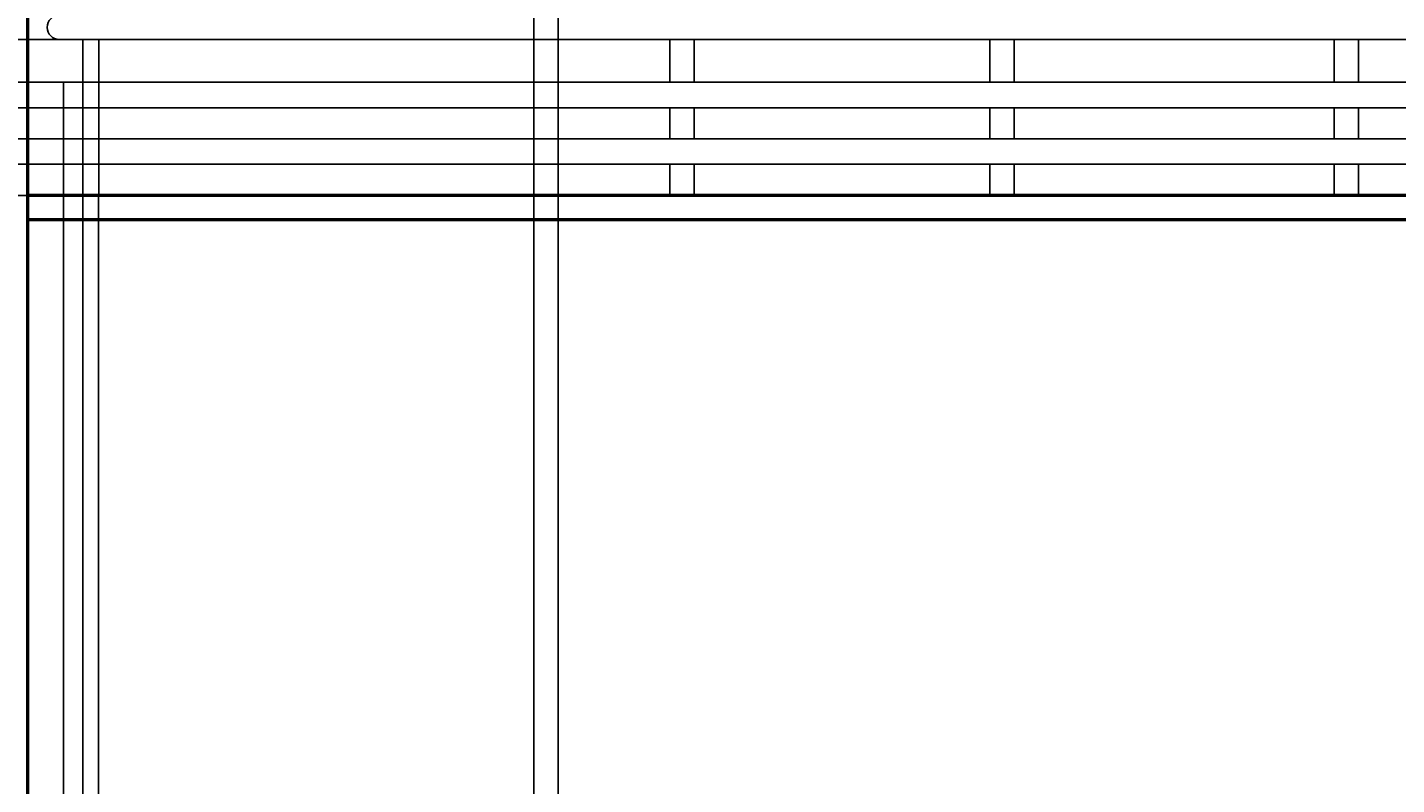
# Model space of a CAD drawing. Units: inches. Extents: x -139 to 346, y 72 to 413.
# Tile 7 of 18: x -47 to 66, y 242 to 305. Entities that reach past the tile are written whole.
import ezdxf

# ---------------------------------------------------------------- set-up
doc = ezdxf.new("R2010")
doc.units = ezdxf.units.IN
doc.header["$MEASUREMENT"] = 0
for name, color, linetype, lineweight in [('A-ANNO-DIMS', 2, 'Continuous', 18), ('A-DOOR', 3, 'Continuous', 25), ('A-ELEV-RAIL', 6, 'Continuous', 25), ('A-WALL', 7, 'Continuous', 50)]:
    doc.layers.add(name, color=color, linetype=linetype, lineweight=lineweight)
doc.styles.get("Standard").update_dxf_attribs({"font": 'arial.ttf'})
doc.dimstyles.get("Standard").update_dxf_attribs({"dimtxt": 0.6875, "dimasz": 0.18, "dimexe": 0.18, "dimexo": 0.0625, "dimgap": 0.09, "dimtad": 0, "dimtih": 1, "dimtoh": 1, "dimdec": 4, "dimzin": 0, "dimdsep": 46, "dimlunit": 4, "dimtxsty": 'Standard', "dimcen": 0.09, "dimadec": 0, "dimazin": 0, "dimtfac": 1, "dimtdec": 4, "dimtofl": 0, "dimtmove": 0, "dimatfit": 3, "dimfxl": 1, "dimtolj": 1, "dimtzin": 0, "dimarcsym": 0})

# ---------------------------------------------------------------- blocks, each defined once
blk = doc.blocks.new('*D44')
at = {"layer": 'A-ANNO-DIMS', "color": 0, "lineweight": -2, "transparency": 16777216}
for p, q in [((5.61, 338.32), (-137.3, 338.32)), ((-137.12, 338.14), (-137.12, 315.13)), ((-137.12, 291.24), (-137.12, 314.25)), ((-47.34, 291.06), (-137.3, 291.06))]:
    blk.add_line(p, q, dxfattribs=at)
at = {"layer": 'A-ANNO-DIMS', "color": 0, "transparency": 16777216}
for points in [[(-137.15, 338.14), (-137.09, 338.14), (-137.12, 338.32)], [(-137.15, 291.24), (-137.09, 291.24), (-137.12, 291.06)]]:
    blk.add_solid(points, dxfattribs=at)
at = {"layer": 'Defpoints', "color": 0, "transparency": 16777216}
for p in [(-137.12, 338.32), (5.67, 338.32), (-47.27, 291.06)]:
    blk.add_point(p, dxfattribs=at)
at = {"layer": 'A-ANNO-DIMS', "color": 0, "transparency": 16777216, "insert": (-137.12, 314.69), "char_height": 0.688, "attachment_point": 5}
blk.add_mtext('\\A1;47.26', dxfattribs=at)
blk = doc.blocks.new('*D68')
at = {"layer": 'A-ANNO-DIMS', "color": 0, "lineweight": -2, "transparency": 16777216}
for p, q in [((-5.54, 207.59), (-5.54, 412.45)), ((-5.36, 412.27), (-4.86, 412.27)), ((-3.72, 412.27), (-4.22, 412.27)), ((-3.54, 205.59), (-3.54, 412.45))]:
    blk.add_line(p, q, dxfattribs=at)
at = {"layer": 'A-ANNO-DIMS', "color": 0, "transparency": 16777216}
for points in [[(-5.36, 412.3), (-5.36, 412.24), (-5.54, 412.27)], [(-3.72, 412.3), (-3.72, 412.24), (-3.54, 412.27)]]:
    blk.add_solid(points, dxfattribs=at)
at = {"layer": 'Defpoints', "color": 0, "transparency": 16777216}
for p in [(-3.54, 412.27), (-5.54, 207.52), (-3.54, 205.52)]:
    blk.add_point(p, dxfattribs=at)
at = {"layer": 'A-ANNO-DIMS', "color": 0, "transparency": 16777216, "insert": (-4.54, 412.27), "char_height": 0.688, "attachment_point": 5}
blk.add_mtext('\\A1;2', dxfattribs=at)
blk = doc.blocks.new('*D89')
at = {"layer": 'A-ANNO-DIMS', "color": 0, "lineweight": -2, "transparency": 16777216}
for p, q in [((62.36, 338.32), (-137.3, 338.32)), ((-137.12, 338.14), (-137.12, 315.13)), ((-137.12, 291.24), (-137.12, 314.25)), ((62.36, 291.06), (-137.3, 291.06))]:
    blk.add_line(p, q, dxfattribs=at)
at = {"layer": 'A-ANNO-DIMS', "color": 0, "transparency": 16777216}
for points in [[(-137.15, 338.14), (-137.09, 338.14), (-137.12, 338.32)], [(-137.15, 291.24), (-137.09, 291.24), (-137.12, 291.06)]]:
    blk.add_solid(points, dxfattribs=at)
at = {"layer": 'Defpoints', "color": 0, "transparency": 16777216}
for p in [(-137.12, 338.32), (62.43, 338.32), (62.43, 291.06)]:
    blk.add_point(p, dxfattribs=at)
at = {"layer": 'A-ANNO-DIMS', "color": 0, "transparency": 16777216, "insert": (-137.12, 314.69), "char_height": 0.688, "attachment_point": 5}
blk.add_mtext('\\A1;47.26', dxfattribs=at)
blk = doc.blocks.new('*D93')
at = {"layer": 'A-ANNO-DIMS', "color": 0, "lineweight": -2, "transparency": 16777216}
for p, q in [((-44.29, 298.23), (-44.29, 72.49)), ((-42.71, 291), (-42.71, 72.49)), ((-44.11, 72.67), (-42.89, 72.67)), ((-42.71, 72.67), (-42.53, 72.67))]:
    blk.add_line(p, q, dxfattribs=at)
at = {"layer": 'A-ANNO-DIMS', "color": 0, "transparency": 16777216}
for points in [[(-44.11, 72.7), (-44.11, 72.64), (-44.29, 72.67)], [(-42.89, 72.7), (-42.89, 72.64), (-42.71, 72.67)]]:
    blk.add_solid(points, dxfattribs=at)
at = {"layer": 'Defpoints', "color": 0, "transparency": 16777216}
for p in [(-44.29, 298.29), (-42.71, 291.06), (-42.71, 72.67)]:
    blk.add_point(p, dxfattribs=at)
at = {"layer": 'A-ANNO-DIMS', "color": 0, "transparency": 16777216, "insert": (-41.58, 72.67), "char_height": 0.688, "attachment_point": 5}
blk.add_mtext('\\A1;1.58', dxfattribs=at)
blk = doc.blocks.new('*D94')
at = {"layer": 'A-ANNO-DIMS', "color": 0, "lineweight": -2, "transparency": 16777216}
for p, q in [((-42.71, 291), (-42.71, 72.49)), ((-41.4, 291), (-41.4, 72.49)), ((-42.53, 72.67), (-41.58, 72.67)), ((-41.4, 72.67), (-41.22, 72.67))]:
    blk.add_line(p, q, dxfattribs=at)
at = {"layer": 'A-ANNO-DIMS', "color": 0, "transparency": 16777216}
for points in [[(-42.53, 72.7), (-42.53, 72.64), (-42.71, 72.67)], [(-41.58, 72.7), (-41.58, 72.64), (-41.4, 72.67)]]:
    blk.add_solid(points, dxfattribs=at)
at = {"layer": 'Defpoints', "color": 0, "transparency": 16777216}
for p in [(-42.71, 291.06), (-41.4, 291.06), (-41.4, 72.67)]:
    blk.add_point(p, dxfattribs=at)
at = {"layer": 'A-ANNO-DIMS', "color": 0, "transparency": 16777216, "insert": (-40.27, 72.67), "char_height": 0.688, "attachment_point": 5}
blk.add_mtext('\\A1;1.32', dxfattribs=at)
blk = doc.blocks.new('*D95')
at = {"layer": 'A-ANNO-DIMS', "color": 0, "lineweight": -2, "transparency": 16777216}
for p, q in [((98.61, 293.63), (-137.3, 293.63)), ((-137.12, 293.45), (-137.12, 292.78)), ((-137.12, 291.24), (-137.12, 291.9)), ((98.61, 291.06), (-137.3, 291.06))]:
    blk.add_line(p, q, dxfattribs=at)
at = {"layer": 'A-ANNO-DIMS', "color": 0, "transparency": 16777216}
for points in [[(-137.15, 293.45), (-137.09, 293.45), (-137.12, 293.63)], [(-137.15, 291.24), (-137.09, 291.24), (-137.12, 291.06)]]:
    blk.add_solid(points, dxfattribs=at)
at = {"layer": 'Defpoints', "color": 0, "transparency": 16777216}
for p in [(-137.12, 293.63), (98.67, 293.63), (98.67, 291.06)]:
    blk.add_point(p, dxfattribs=at)
at = {"layer": 'A-ANNO-DIMS', "color": 0, "transparency": 16777216, "insert": (-137.12, 292.34), "char_height": 0.688, "attachment_point": 5}
blk.add_mtext('\\A1;2.566', dxfattribs=at)
blk = doc.blocks.new('*D96')
at = {"layer": 'A-ANNO-DIMS', "color": 0, "lineweight": -2, "transparency": 16777216}
for p, q in [((98.61, 295.74), (-137.3, 295.74)), ((-137.12, 295.56), (-137.12, 295.12)), ((98.61, 293.63), (-137.3, 293.63)), ((-137.12, 293.81), (-137.12, 294.25))]:
    blk.add_line(p, q, dxfattribs=at)
at = {"layer": 'A-ANNO-DIMS', "color": 0, "transparency": 16777216}
for points in [[(-137.15, 295.56), (-137.09, 295.56), (-137.12, 295.74)], [(-137.15, 293.81), (-137.09, 293.81), (-137.12, 293.63)]]:
    blk.add_solid(points, dxfattribs=at)
at = {"layer": 'Defpoints', "color": 0, "transparency": 16777216}
for p in [(-137.12, 295.74), (98.67, 295.74), (98.67, 293.63)]:
    blk.add_point(p, dxfattribs=at)
at = {"layer": 'A-ANNO-DIMS', "color": 0, "transparency": 16777216, "insert": (-137.12, 294.68), "char_height": 0.688, "attachment_point": 5}
blk.add_mtext('\\A1;2.11', dxfattribs=at)
blk = doc.blocks.new('*D97')
at = {"layer": 'A-ANNO-DIMS', "color": 0, "lineweight": -2, "transparency": 16777216}
for p, q in [((98.61, 298.29), (-137.3, 298.29)), ((-137.12, 298.11), (-137.12, 297.46)), ((98.61, 295.74), (-137.3, 295.74)), ((-137.12, 295.92), (-137.12, 296.57))]:
    blk.add_line(p, q, dxfattribs=at)
at = {"layer": 'A-ANNO-DIMS', "color": 0, "transparency": 16777216}
for points in [[(-137.15, 298.11), (-137.09, 298.11), (-137.12, 298.29)], [(-137.15, 295.92), (-137.09, 295.92), (-137.12, 295.74)]]:
    blk.add_solid(points, dxfattribs=at)
at = {"layer": 'Defpoints', "color": 0, "transparency": 16777216}
for p in [(-137.12, 298.29), (98.67, 298.29), (98.67, 295.74)]:
    blk.add_point(p, dxfattribs=at)
at = {"layer": 'A-ANNO-DIMS', "color": 0, "transparency": 16777216, "insert": (-137.12, 297.02), "char_height": 0.688, "attachment_point": 5}
blk.add_mtext('\\A1;2.555', dxfattribs=at)
blk = doc.blocks.new('*D98')
at = {"layer": 'A-ANNO-DIMS', "color": 0, "lineweight": -2, "transparency": 16777216}
for p, q in [((98.61, 300.4), (-137.3, 300.4)), ((-137.12, 300.22), (-137.12, 299.78)), ((98.61, 298.29), (-137.3, 298.29)), ((-137.12, 298.47), (-137.12, 298.91))]:
    blk.add_line(p, q, dxfattribs=at)
at = {"layer": 'A-ANNO-DIMS', "color": 0, "transparency": 16777216}
for points in [[(-137.15, 300.22), (-137.09, 300.22), (-137.12, 300.4)], [(-137.15, 298.47), (-137.09, 298.47), (-137.12, 298.29)]]:
    blk.add_solid(points, dxfattribs=at)
at = {"layer": 'Defpoints', "color": 0, "transparency": 16777216}
for p in [(-137.12, 300.4), (98.67, 300.4), (98.67, 298.29)]:
    blk.add_point(p, dxfattribs=at)
at = {"layer": 'A-ANNO-DIMS', "color": 0, "transparency": 16777216, "insert": (-137.12, 299.35), "char_height": 0.688, "attachment_point": 5}
blk.add_mtext('\\A1;2.11', dxfattribs=at)
blk = doc.blocks.new('*D99')
at = {"layer": 'A-ANNO-DIMS', "color": 0, "lineweight": -2, "transparency": 16777216}
for p, q in [((98.61, 303.92), (-137.3, 303.92)), ((-137.12, 303.74), (-137.12, 302.6)), ((-137.12, 300.58), (-137.12, 301.72)), ((98.61, 300.4), (-137.3, 300.4))]:
    blk.add_line(p, q, dxfattribs=at)
at = {"layer": 'A-ANNO-DIMS', "color": 0, "transparency": 16777216}
for points in [[(-137.15, 303.74), (-137.09, 303.74), (-137.12, 303.92)], [(-137.15, 300.58), (-137.09, 300.58), (-137.12, 300.4)]]:
    blk.add_solid(points, dxfattribs=at)
at = {"layer": 'Defpoints', "color": 0, "transparency": 16777216}
for p in [(-137.12, 303.92), (98.67, 303.92), (98.67, 300.4)]:
    blk.add_point(p, dxfattribs=at)
at = {"layer": 'A-ANNO-DIMS', "color": 0, "transparency": 16777216, "insert": (-137.12, 302.16), "char_height": 0.688, "attachment_point": 5}
blk.add_mtext('\\A1;3.516', dxfattribs=at)
blk = doc.blocks.new('*D100')
at = {"layer": 'A-ANNO-DIMS', "color": 0, "lineweight": -2, "transparency": 16777216}
for p, q in [((98.61, 305.92), (-137.3, 305.92)), ((-137.12, 305.74), (-137.12, 305.36)), ((98.61, 303.92), (-137.3, 303.92)), ((-137.12, 304.1), (-137.12, 304.49))]:
    blk.add_line(p, q, dxfattribs=at)
at = {"layer": 'A-ANNO-DIMS', "color": 0, "transparency": 16777216}
for points in [[(-137.15, 305.74), (-137.09, 305.74), (-137.12, 305.92)], [(-137.15, 304.1), (-137.09, 304.1), (-137.12, 303.92)]]:
    blk.add_solid(points, dxfattribs=at)
at = {"layer": 'Defpoints', "color": 0, "transparency": 16777216}
for p in [(-137.12, 305.92), (98.67, 305.92), (98.67, 303.92)]:
    blk.add_point(p, dxfattribs=at)
at = {"layer": 'A-ANNO-DIMS', "color": 0, "transparency": 16777216, "insert": (-137.12, 304.92), "char_height": 0.688, "attachment_point": 5}
blk.add_mtext('\\A1;2', dxfattribs=at)

msp = doc.modelspace()

# ---------------------------------------------------------------- linework, layer by layer
at = {"layer": 'A-DOOR'}
for p, q in [((32.0494, 303.9205), (32.0494, 300.4047)), ((34.0494, 303.9205), (34.0494, 300.4047)), ((32.0494, 298.293), (32.0494, 295.7379)), ((34.0494, 298.293), (34.0494, 295.7379)), ((32.0494, 293.6263), (32.0494, 291.0604)), ((34.0494, 293.6263), (34.0494, 291.0604))]:
    msp.add_line(p, q, dxfattribs=at)
for points in [[(5.6729, 303.9205), (5.6729, 300.4047)], [(7.6729, 303.9205), (7.6729, 300.4047)], [(60.4258, 300.4047), (60.4258, 303.9205)], [(62.4258, 300.4047), (62.4258, 303.9205)], [(5.6729, 298.293), (5.6729, 295.7379)], [(7.6729, 298.293), (7.6729, 295.7379)], [(60.4258, 295.7379), (60.4258, 298.293)], [(62.4258, 295.7379), (62.4258, 298.293)], [(5.6729, 293.6263), (5.6729, 291.0604)], [(7.6729, 293.6263), (7.6729, 291.0604), (60.4258, 291.0604), (60.4258, 293.6263)], [(62.4258, 291.0604), (62.4258, 293.6263)], [(5.6729, 289.0604), (62.4258, 289.0604)]]:
    msp.add_lwpolyline(points, dxfattribs=at)
at = {"layer": 'A-ELEV-RAIL'}
for p, q in [((-44.6423, 303.9205), (110.3243, 303.9205)), ((-42.7149, 300.3938), (-42.7149, 303.9205)), ((-42.7149, 303.9205), (-41.3972, 303.9205)), ((-41.3972, 303.9205), (-41.3972, 300.3938)), ((-42.7149, 291.0604), (-42.7149, 300.3938)), ((-42.7149, 300.3938), (-41.3972, 300.3938)), ((-41.3972, 300.3938), (-41.3972, 291.0604))]:
    msp.add_line(p, q, dxfattribs=at)
for points in [[(-44.2923, 300.4047), (110.3243, 300.4047), (110.3243, 298.293), (-44.2923, 298.293)], [(-44.2923, 295.7379), (110.3243, 295.7379), (110.3243, 293.6263), (-44.2923, 293.6263)]]:
    msp.add_lwpolyline(points, close=True, dxfattribs=at)
msp.add_arc((-44.6423, 304.9205), 1, 90, 270, dxfattribs=at)
at = {"layer": 'A-WALL'}
for p, q in [((-47.2734, 382.9748), (-47.2734, 291.0604)), ((112.6506, 291.0604), (-47.2734, 291.0604)), ((-47.2734, 291.0604), (-47.2734, 94.9748)), ((112.6506, 289.0604), (-47.2734, 289.0604))]:
    msp.add_line(p, q, dxfattribs=at)

# ---------------------------------------------------------------- dimensions: what is measured, and where the dimension line sits
at = {"layer": 'A-ANNO-DIMS'}
for base, p1, p2, override, picture, middle in [((-3.5402, 412.2748), (-5.5402, 207.5243), (-3.5402, 205.5243), {"dimdec": 0, "dimlfac": 1, "dimrnd": 0, "dimzin": 0, "dimdsep": 46, "dimlunit": 2}, '*D68', (-4.5402, 412.2748)), ((-42.7149, 72.6748), (-44.2923, 298.293), (-42.7149, 291.0604), {"dimdec": 2, "dimlfac": 1, "dimrnd": 0, "dimzin": 0, "dimdsep": 46, "dimlunit": 2}, '*D93', (-41.5836, 72.6748)), ((-41.3972, 72.6748), (-42.7149, 291.0604), (-41.3972, 291.0604), {"dimdec": 2, "dimlfac": 1, "dimrnd": 0, "dimzin": 0, "dimdsep": 46, "dimlunit": 2}, '*D94', (-40.2702, 72.6748))]:
    dim = msp.add_linear_dim(base=base, p1=p1, p2=p2, dimstyle='Standard', override=override, dxfattribs=at)
    dim.commit()
    dim.dimension.update_dxf_attribs({"geometry": picture, "text_midpoint": middle})
for base, p1, p2, override, picture, middle in [((-137.1237, 338.3217), (-47.2734, 291.0604), (5.6729, 338.3217), {"dimdec": 2, "dimlfac": 1, "dimrnd": 0, "dimzin": 0, "dimdsep": 46, "dimlunit": 2}, '*D44', (-137.1237, 314.691)), ((-137.1237, 338.3217), (62.4258, 291.0604), (62.4258, 338.3217), {"dimdec": 2, "dimlfac": 1, "dimrnd": 0, "dimzin": 0, "dimdsep": 46, "dimlunit": 2}, '*D89', (-137.1237, 314.691)), ((-137.1237, 305.9205), (98.6724, 303.9205), (98.6724, 305.9205), {"dimdec": 0, "dimlfac": 1, "dimrnd": 0, "dimzin": 0, "dimdsep": 46, "dimlunit": 2}, '*D100', (-137.1237, 304.9205)), ((-137.1237, 303.9205), (98.6724, 300.4047), (98.6724, 303.9205), {"dimdec": 3, "dimlfac": 1, "dimrnd": 0, "dimzin": 0, "dimdsep": 46, "dimlunit": 2}, '*D99', (-137.1237, 302.1626)), ((-137.1237, 300.4047), (98.6724, 298.293), (98.6724, 300.4047), {"dimdec": 2, "dimlfac": 1, "dimrnd": 0, "dimzin": 0, "dimdsep": 46, "dimlunit": 2}, '*D98', (-137.1237, 299.3488)), ((-137.1237, 298.293), (98.6724, 295.7379), (98.6724, 298.293), {"dimdec": 3, "dimlfac": 1, "dimrnd": 0, "dimzin": 0, "dimdsep": 46, "dimlunit": 2}, '*D97', (-137.1237, 297.0155)), ((-137.1237, 295.7379), (98.6724, 293.6263), (98.6724, 295.7379), {"dimdec": 2, "dimlfac": 1, "dimrnd": 0, "dimzin": 0, "dimdsep": 46, "dimlunit": 2}, '*D96', (-137.1237, 294.6821)), ((-137.1237, 293.6263), (98.6724, 291.0604), (98.6724, 293.6263), {"dimdec": 3, "dimlfac": 1, "dimrnd": 0, "dimzin": 0, "dimdsep": 46, "dimlunit": 2}, '*D95', (-137.1237, 292.3433))]:
    dim = msp.add_linear_dim(base=base, p1=p1, p2=p2, angle=90, dimstyle='Standard', override=override, dxfattribs=at)
    dim.commit()
    dim.dimension.update_dxf_attribs({"geometry": picture, "text_midpoint": middle})

doc.saveas('drawing.dxf')
